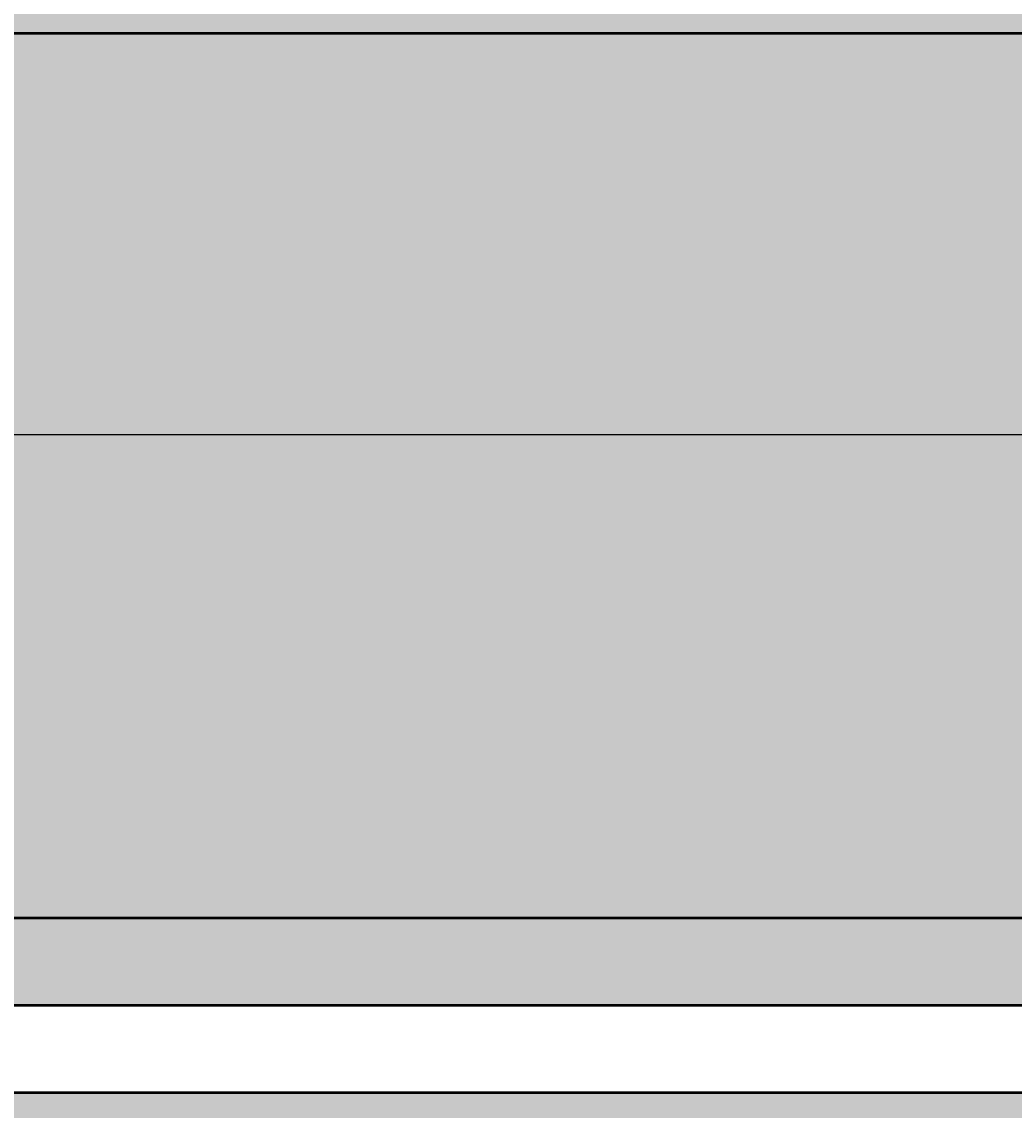
# Model space of a CAD drawing. Units: inches. Extents: x -12 to 334, y -10 to 186.
# Tile 36 of 77: x 106 to 129, y 65 to 90. Entities that reach past the tile are written whole.
import ezdxf

# ---------------------------------------------------------------- set-up
doc = ezdxf.new("R2010")
doc.units = ezdxf.units.IN
doc.header["$MEASUREMENT"] = 0
for name, color, linetype, lineweight in [('M-DIMS', 2, 'Continuous', 18), ('M-EQPM', 7, 'Continuous', 50), ('M-EQPM-PATT', 8, 'Continuous', 18)]:
    doc.layers.add(name, color=color, linetype=linetype, lineweight=lineweight)
doc.styles.get("Standard").update_dxf_attribs({"font": 'arial.ttf'})
doc.dimstyles.get("Standard").update_dxf_attribs({"dimtxt": 0.18, "dimasz": 0.18, "dimexe": 0.18, "dimexo": 0.0625, "dimgap": 0.09, "dimtad": 0, "dimtih": 1, "dimtoh": 1, "dimdec": 4, "dimzin": 0, "dimdsep": 46, "dimtxsty": 'Standard', "dimcen": 0.09, "dimadec": 0, "dimazin": 0, "dimtfac": 1, "dimtdec": 4, "dimtofl": 0, "dimtmove": 0, "dimatfit": 3, "dimfxl": 1, "dimtolj": 1, "dimtzin": 0, "dimarcsym": 0})

# ---------------------------------------------------------------- blocks, each defined once
blk = doc.blocks.new('*D1')
at = {"layer": 'Defpoints', "color": 0, "transparency": 16777216}
for p in [(281.426, 91.899), (3.376, 80.692), (281.426, 14.304)]:
    blk.add_point(p, dxfattribs=at)
at = {"layer": 'M-DIMS', "color": 0, "lineweight": -2, "transparency": 16777216}
for p, q in [((281.426, 91.836), (281.426, 14.124)), ((3.376, 80.629), (3.376, 14.124)), ((3.556, 14.304), (141.935, 14.304)), ((281.246, 14.304), (142.867, 14.304))]:
    blk.add_line(p, q, dxfattribs=at)
at = {"layer": 'M-DIMS', "color": 0, "transparency": 16777216}
for points in [[(3.556, 14.334), (3.556, 14.274), (3.376, 14.304)], [(281.246, 14.334), (281.246, 14.274), (281.426, 14.304)]]:
    blk.add_solid(points, dxfattribs=at)
at = {"layer": 'M-DIMS', "color": 0, "transparency": 16777216, "insert": (142.401, 14.304), "char_height": 0.18, "attachment_point": 5}
blk.add_mtext('\\A1;278.05', dxfattribs=at)
blk = doc.blocks.new('*D17')
at = {"layer": 'Defpoints', "color": 0, "transparency": 16777216}
for p in [(106.177, 102.896), (105.892, 56.321), (295.976, 56.321)]:
    blk.add_point(p, dxfattribs=at)
at = {"layer": 'M-DIMS', "color": 0, "lineweight": -2, "transparency": 16777216}
for p, q in [((106.24, 102.896), (296.156, 102.896)), ((295.976, 102.716), (295.976, 79.79)), ((295.976, 56.501), (295.976, 79.426)), ((105.954, 56.321), (296.156, 56.321))]:
    blk.add_line(p, q, dxfattribs=at)
at = {"layer": 'M-DIMS', "color": 0, "transparency": 16777216}
for points in [[(295.946, 102.716), (296.006, 102.716), (295.976, 102.896)], [(295.946, 56.501), (296.006, 56.501), (295.976, 56.321)]]:
    blk.add_solid(points, dxfattribs=at)
at = {"layer": 'M-DIMS', "color": 0, "transparency": 16777216, "insert": (295.976, 79.608), "char_height": 0.18, "attachment_point": 5}
blk.add_mtext('\\A1;46.575', dxfattribs=at)
blk = doc.blocks.new('*D35')
at = {"layer": 'Defpoints', "color": 0, "transparency": 16777216}
for p in [(216.428, 98.108), (-11.174, 61.105), (216.428, 61.105)]:
    blk.add_point(p, dxfattribs=at)
at = {"layer": 'M-DIMS', "color": 0, "lineweight": -2, "transparency": 16777216}
for p, q in [((216.365, 98.108), (-11.354, 98.108)), ((-11.174, 97.928), (-11.174, 79.788)), ((-11.174, 61.285), (-11.174, 79.424)), ((216.365, 61.105), (-11.354, 61.105))]:
    blk.add_line(p, q, dxfattribs=at)
at = {"layer": 'M-DIMS', "color": 0, "transparency": 16777216}
for points in [[(-11.204, 97.928), (-11.144, 97.928), (-11.174, 98.108)], [(-11.204, 61.285), (-11.144, 61.285), (-11.174, 61.105)]]:
    blk.add_solid(points, dxfattribs=at)
at = {"layer": 'M-DIMS', "color": 0, "transparency": 16777216, "insert": (-11.174, 79.606), "char_height": 0.18, "attachment_point": 5}
blk.add_mtext('\\A1;37', dxfattribs=at)
blk = doc.blocks.new('*D39')
at = {"layer": 'Defpoints', "color": 0, "transparency": 16777216}
for p in [(279.726, 80.692), (-11.174, 45.854), (269.381, 45.854)]:
    blk.add_point(p, dxfattribs=at)
at = {"layer": 'M-DIMS', "color": 0, "lineweight": -2, "transparency": 16777216}
for p, q in [((279.664, 80.692), (-11.354, 80.692)), ((-11.174, 80.512), (-11.174, 63.455)), ((-11.174, 46.034), (-11.174, 63.091)), ((269.318, 45.854), (-11.354, 45.854))]:
    blk.add_line(p, q, dxfattribs=at)
at = {"layer": 'M-DIMS', "color": 0, "transparency": 16777216}
for points in [[(-11.204, 80.512), (-11.144, 80.512), (-11.174, 80.692)], [(-11.204, 46.034), (-11.144, 46.034), (-11.174, 45.854)]]:
    blk.add_solid(points, dxfattribs=at)
at = {"layer": 'M-DIMS', "color": 0, "transparency": 16777216, "insert": (-11.174, 63.273), "char_height": 0.18, "attachment_point": 5}
blk.add_mtext('\\A1;34.84', dxfattribs=at)

msp = doc.modelspace()

# ---------------------------------------------------------------- hatches: boundary and pattern name
at = {"layer": 'M-EQPM-PATT'}
h = msp.add_hatch(color=256, dxfattribs=at)
h.set_gradient(color1=(205, 32, 39), color2=(205, 32, 39), tint=1)
h.paths.add_polyline_path([(64.5, 80.754), (64.5, 89.8963), (226.6083, 89.8963, -1), (226.6083, 69.6117), (64.5, 69.6117), (64.5, 78.754), (4.4744, 78.754, 0.384914), (23.5807, 61.4872), (37.1002, 61.4872), (37.1002, 33.6752), (53.1002, 33.6752), (53.1002, 61.4872), (64.5, 61.4872), (64.5, 63.6117), (226.6083, 63.6117, 1), (226.6083, 95.8963), (64.5, 95.8963), (64.5, 99.8958), (53.1002, 99.8958), (53.1002, 127.7078), (37.1002, 127.7078), (37.1002, 99.8958), (23.5807, 99.8958, 0.4132606), (4.3766, 80.754)])
h.paths.add_polyline_path([(64.5, 91.8963), (64.5, 93.8963), (226.6083, 93.8963, -1), (226.6083, 65.6117), (64.5, 65.6117), (64.5, 67.6117), (226.6083, 67.6117, 1), (226.6083, 91.8963)], flags=16)
h = msp.add_hatch(color=256, dxfattribs=at)
h.set_gradient(color1=(94, 103, 175), color2=(94, 103, 175), tint=1)
h.paths.add_polyline_path([(129.093, 89.8963), (86.8879, 89.8963), (86.8879, 69.6117), (129.093, 69.6117)], flags=17)
h.paths.add_polyline_path([(170.9079, 89.8963), (130.8573, 89.8963), (130.8573, 69.6117), (170.9079, 69.6117)], flags=17)
h.paths.add_polyline_path([(216.4278, 89.8963), (172.6722, 89.8963), (172.6722, 69.6117), (216.4278, 69.6117)], flags=17)
h.paths.add_polyline_path([(245.9354, 82.6969), (247.9354, 82.6969), (247.9354, 46.8541), (268.3808, 46.8541, 0.0998398), (279.7263, 80.6915), (251.9801, 80.6915, 0.4142136), (231.7758, 100.8958), (84.7229, 100.8958), (84.7229, 109.0583), (83.7229, 109.0583), (83.7229, 95.8963), (129.093, 95.8963), (129.093, 98.1081), (130.8573, 98.1081), (130.8573, 95.8963), (170.9079, 95.8963), (170.9079, 98.1081), (172.6722, 98.1081), (172.6722, 95.8963), (216.4278, 95.8963), (216.4278, 98.1081), (218.1922, 98.1081), (218.1922, 95.8963), (226.6083, 95.8963, -1), (226.6083, 63.6117), (218.1922, 63.6117), (218.1922, 61.1045), (216.4278, 61.1045), (216.4278, 63.6117), (172.6722, 63.6117), (172.6722, 61.1045), (170.9079, 61.1045), (170.9079, 63.6117), (130.8573, 63.6117), (130.8573, 61.1045), (129.093, 61.1045), (129.093, 63.6117), (87.8879, 63.6117), (87.8879, 56.3205), (105.8919, 56.3205), (105.8919, 28.8541), (115.8919, 28.8541), (115.8919, 46.8541), (222.5761, 46.8541), (222.5761, 30.8541), (232.5761, 30.8541), (232.5761, 46.8541), (245.9354, 46.8541)])
h.paths.add_polyline_path([(86.8879, 89.8963), (75.9244, 89.8963), (75.9244, 69.6117), (86.8879, 69.6117)])
h.paths.add_polyline_path([(83.7229, 109.0583), (75.9244, 109.0583), (75.9244, 95.8963), (83.7229, 95.8963)])
h.paths.add_polyline_path([(226.6083, 89.8963), (218.1922, 89.8963), (218.1922, 69.6117), (226.6083, 69.6117, 1)], flags=17)

# ---------------------------------------------------------------- linework, layer by layer
at = {"layer": 'M-EQPM'}
for points in [[(64.5, 65.6117), (226.6083, 65.6117, 1), (226.6083, 93.8963), (64.5, 93.8963)], [(64.5, 67.6117), (226.6083, 67.6117, 1), (226.6083, 91.8963), (64.5, 91.8963)], [(64.5, 69.6117), (226.6083, 69.6117, 1), (226.6083, 89.8963), (64.5, 89.8963)]]:
    msp.add_lwpolyline(points, format="xyb", dxfattribs=at)

# ---------------------------------------------------------------- dimensions: what is measured, and where the dimension line sits
at = {"layer": 'M-DIMS'}
for base, p1, p2, override, picture, middle in [((295.9756, 56.3205), (106.1771, 102.8958), (105.8919, 56.3205), {"dimdec": 3, "dimlfac": 1, "dimrnd": 0, "dimzin": 0, "dimdsep": 46, "dimlunit": 2}, '*D17', (295.9756, 79.6082)), ((-11.1736, 61.1045), (216.4278, 98.1081), (216.4278, 61.1045), {"dimdec": 0, "dimlfac": 1, "dimrnd": 0, "dimzin": 0, "dimdsep": 46, "dimlunit": 2}, '*D35', (-11.1735, 79.6063)), ((-11.1736, 45.8541), (279.7263, 80.6915), (269.3808, 45.8541), {"dimdec": 2, "dimlfac": 1, "dimrnd": 0, "dimzin": 0, "dimdsep": 46, "dimlunit": 2}, '*D39', (-11.1735, 63.2728))]:
    dim = msp.add_linear_dim(base=base, p1=p1, p2=p2, angle=90, dimstyle='Standard', override=override, dxfattribs=at)
    dim.commit()
    dim.dimension.update_dxf_attribs({"geometry": picture, "text_midpoint": middle})
dim = msp.add_linear_dim(base=(281.4256, 14.3041), p1=(3.3765, 80.6915), p2=(281.4256, 91.8988), dimstyle='Standard', override={"dimdec": 2, "dimlfac": 1, "dimrnd": 0, "dimzin": 0, "dimdsep": 46, "dimlunit": 2}, dxfattribs=at)
dim.commit()
dim.dimension.update_dxf_attribs({"geometry": '*D1', "text_midpoint": (142.401, 14.3041)})

doc.saveas('drawing.dxf')
